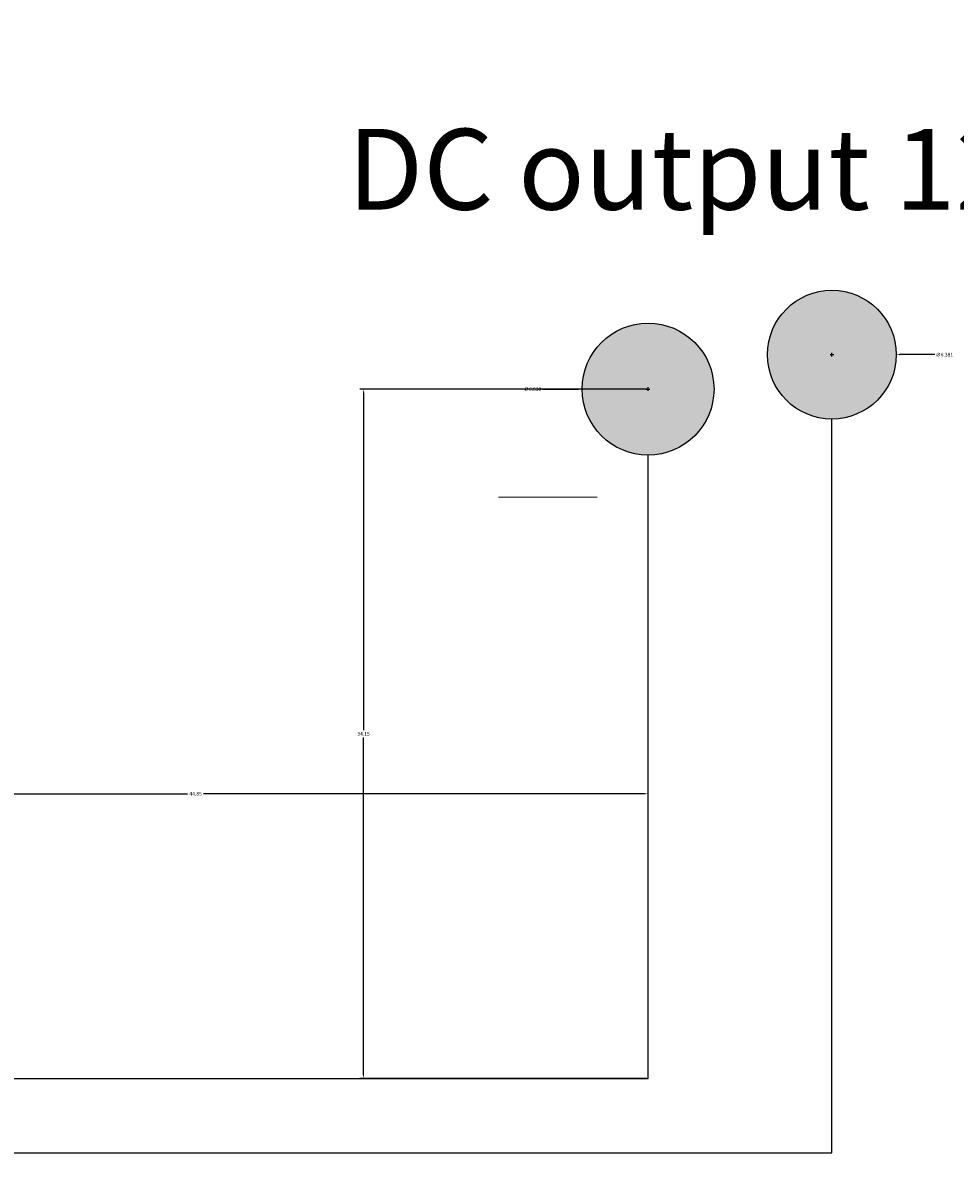
# Model space of a CAD drawing. Units: millimetres. Extents: x -8 to 285, y 5 to 221.
# Tile 9 of 30: x 84 to 130, y 56 to 113. Entities that reach past the tile are written whole.
import ezdxf

# ---------------------------------------------------------------- set-up
doc = ezdxf.new("R2010")
doc.units = ezdxf.units.MM
for name, color, linetype, lineweight in [('A-ANNO-DIMS', 2, 'Continuous', 18), ('E-ANNO-SYMB', 7, 'Continuous', 18), ('E-ANNO-TEXT', 7, 'Continuous', 18), ('E-EQPM-PATT', 252, 'Continuous', 13), ('E-POWR-DC-NEG', 3, 'Continuous', 25), ('E-POWR-LOAD', 7, 'Continuous', 25)]:
    doc.layers.add(name, color=color, linetype=linetype, lineweight=lineweight)
doc.layers.add('E-POWR-DC-POS', color=30, linetype='Continuous', lineweight=25, true_color=0xf26722)
doc.styles.get("Standard").update_dxf_attribs({"font": 'arial.ttf'})
doc.dimstyles.get("Standard").update_dxf_attribs({"dimtxt": 0.18, "dimasz": 0.18, "dimexe": 0.18, "dimexo": 0.0625, "dimgap": 0.09, "dimtad": 0, "dimtih": 1, "dimtoh": 1, "dimdec": 4, "dimzin": 0, "dimdsep": 46, "dimtxsty": 'Standard', "dimcen": 0.09, "dimadec": 0, "dimazin": 0, "dimtfac": 1, "dimtdec": 4, "dimtofl": 0, "dimtmove": 0, "dimatfit": 3, "dimfxl": 1, "dimtolj": 1, "dimtzin": 0, "dimarcsym": 0})

# ---------------------------------------------------------------- blocks, each defined once
blk = doc.blocks.new('*D10')
at = {"layer": 'A-ANNO-DIMS', "color": 0, "lineweight": -2, "transparency": 16777216}
for p, q in [((145.103, 206.457), (-7.608, 206.457)), ((-7.428, 206.277), (-7.428, 113.161)), ((-7.428, 19.682), (-7.428, 112.797)), ((30.453, 19.502), (-7.608, 19.502))]:
    blk.add_line(p, q, dxfattribs=at)
at = {"layer": 'A-ANNO-DIMS', "color": 0, "transparency": 16777216}
for points in [[(-7.458, 206.277), (-7.398, 206.277), (-7.428, 206.457)], [(-7.458, 19.682), (-7.398, 19.682), (-7.428, 19.502)]]:
    blk.add_solid(points, dxfattribs=at)
at = {"layer": 'Defpoints', "color": 0, "transparency": 16777216}
for p in [(-7.428, 206.457), (145.165, 206.457), (30.516, 19.502)]:
    blk.add_point(p, dxfattribs=at)
at = {"layer": 'A-ANNO-DIMS', "color": 0, "transparency": 16777216, "insert": (-7.428, 112.979), "char_height": 0.18, "attachment_point": 5}
blk.add_mtext('\\A1;186.95', dxfattribs=at)
blk = doc.blocks.new('*D25')
at = {"layer": 'A-ANNO-DIMS', "color": 0, "lineweight": -2, "transparency": 16777216}
for p, q in [((70.172, 60.759), (70.172, 74.977)), ((70.352, 74.797), (92.199, 74.797)), ((114.842, 74.797), (92.995, 74.797)), ((115.022, 60.759), (115.022, 74.977))]:
    blk.add_line(p, q, dxfattribs=at)
at = {"layer": 'A-ANNO-DIMS', "color": 0, "transparency": 16777216}
for points in [[(70.352, 74.827), (70.352, 74.767), (70.172, 74.797)], [(114.842, 74.827), (114.842, 74.767), (115.022, 74.797)]]:
    blk.add_solid(points, dxfattribs=at)
at = {"layer": 'Defpoints', "color": 0, "transparency": 16777216}
for p in [(115.022, 74.797), (70.172, 60.697), (115.022, 60.697)]:
    blk.add_point(p, dxfattribs=at)
at = {"layer": 'A-ANNO-DIMS', "color": 0, "transparency": 16777216, "insert": (92.597, 74.797), "char_height": 0.18, "attachment_point": 5}
blk.add_mtext('\\A1;44.85', dxfattribs=at)
blk = doc.blocks.new('*D26')
at = {"layer": 'A-ANNO-DIMS', "color": 0, "lineweight": -2, "transparency": 16777216}
for p, q in [((114.96, 94.844), (100.742, 94.844)), ((100.922, 94.664), (100.922, 77.953)), ((100.922, 60.877), (100.922, 77.589)), ((114.96, 60.697), (100.742, 60.697))]:
    blk.add_line(p, q, dxfattribs=at)
at = {"layer": 'A-ANNO-DIMS', "color": 0, "transparency": 16777216}
for points in [[(100.892, 94.664), (100.952, 94.664), (100.922, 94.844)], [(100.892, 60.877), (100.952, 60.877), (100.922, 60.697)]]:
    blk.add_solid(points, dxfattribs=at)
at = {"layer": 'Defpoints', "color": 0, "transparency": 16777216}
for p in [(100.922, 94.844), (115.022, 94.844), (115.022, 60.697)]:
    blk.add_point(p, dxfattribs=at)
at = {"layer": 'A-ANNO-DIMS', "color": 0, "transparency": 16777216, "insert": (100.922, 77.771), "char_height": 0.18, "attachment_point": 5}
blk.add_mtext('\\A1;34.15', dxfattribs=at)
blk = doc.blocks.new('*D35')
at = {"layer": 'A-ANNO-DIMS', "color": 0, "lineweight": -2, "transparency": 16777216}
for p, q in [((109.792, 94.844), (111.573, 94.844)), ((114.932, 94.844), (115.112, 94.844)), ((115.022, 94.754), (115.022, 94.934))]:
    blk.add_line(p, q, dxfattribs=at)
at = {"layer": 'A-ANNO-DIMS', "color": 0, "transparency": 16777216}
blk.add_solid([(111.573, 94.874), (111.573, 94.814), (111.753, 94.844)], dxfattribs=at)
at = {"layer": 'Defpoints', "color": 0, "transparency": 16777216}
for p in [(111.753, 94.844), (118.292, 94.845)]:
    blk.add_point(p, dxfattribs=at)
at = {"layer": 'A-ANNO-DIMS', "color": 0, "transparency": 16777216, "insert": (109.3, 94.844), "char_height": 0.18, "attachment_point": 5}
blk.add_mtext('\\A1;∅6.538', dxfattribs=at)
blk = doc.blocks.new('*D36')
at = {"layer": 'A-ANNO-DIMS', "color": 0, "lineweight": -2, "transparency": 16777216}
for p, q in [((124.044, 96.551), (124.224, 96.551)), ((124.134, 96.461), (124.134, 96.641)), ((129.239, 96.551), (127.504, 96.551))]:
    blk.add_line(p, q, dxfattribs=at)
at = {"layer": 'A-ANNO-DIMS', "color": 0, "transparency": 16777216}
blk.add_solid([(127.504, 96.581), (127.504, 96.521), (127.324, 96.551)], dxfattribs=at)
at = {"layer": 'Defpoints', "color": 0, "transparency": 16777216}
for p in [(120.944, 96.552), (127.324, 96.551)]:
    blk.add_point(p, dxfattribs=at)
at = {"layer": 'A-ANNO-DIMS', "color": 0, "transparency": 16777216, "insert": (129.713, 96.551), "char_height": 0.18, "attachment_point": 5}
blk.add_mtext('\\A1;∅6.381', dxfattribs=at)

msp = doc.modelspace()

# ---------------------------------------------------------------- hatches: boundary and pattern name
at = {"layer": 'E-EQPM-PATT'}
h = msp.add_hatch(color=256, dxfattribs=at)
h.set_gradient(color1=(248, 153, 30), color2=(248, 153, 30), tint=1)
h.paths.add_polyline_path([(111.7534, 94.8444, 1), (118.2915, 94.8444, 1)])
h.paths.add_polyline_path([(127.3244, 96.5513, 1), (120.9436, 96.5513, 1)])
h = msp.add_hatch(color=256, dxfattribs=at)
h.set_gradient(color1=(0, 255, 0), color2=(0, 255, 0), tint=1)
h.paths.add_polyline_path([(118.2915, 94.8444, 1), (111.7534, 94.8444, 1)])

# ---------------------------------------------------------------- linework, layer by layer
at = {"layer": 'E-ANNO-SYMB'}
msp.add_line((107.608, 89.4839), (112.5018, 89.4839), dxfattribs=at)
at = {"layer": 'E-POWR-DC-NEG'}
msp.add_lwpolyline([(70.1717, 67.9064), (70.1717, 60.6968), (115.0224, 60.6968), (115.0224, 91.5754)], dxfattribs=at)
at = {"layer": 'E-POWR-DC-POS'}
msp.add_lwpolyline([(64.1717, 67.9064), (64.1717, 57.0172), (124.134, 57.0172), (124.134, 93.361)], dxfattribs=at)
at = {"layer": 'E-POWR-LOAD'}
for centre, radius in [((124.134, 96.5513), 3.1904), ((115.0224, 94.8444), 3.2691)]:
    msp.add_circle(centre, radius, dxfattribs=at)

# ---------------------------------------------------------------- texts
at = {"layer": 'E-ANNO-TEXT', "insert": (100.1263, 107.7354), "char_height": 4, "attachment_point": 1}
msp.add_mtext_dynamic_manual_height_columns('DC output 12v DC load', width=65.111825, gutter_width=12.5, heights=[0], dxfattribs=at)

# ---------------------------------------------------------------- dimensions: what is measured, and where the dimension line sits
at = {"layer": 'A-ANNO-DIMS'}
for base, p1, p2, picture, middle in [((-7.4275, 206.4568), (30.516, 19.502), (145.1651, 206.4568), '*D10', (-7.4275, 112.9794)), ((100.9224, 94.8444), (115.0224, 60.6968), (115.0224, 94.8444), '*D26', (100.9224, 77.7706))]:
    dim = msp.add_linear_dim(base=base, p1=p1, p2=p2, angle=90, dimstyle='Standard', override={"dimdec": 2, "dimlfac": 1, "dimrnd": 0, "dimzin": 0, "dimdsep": 46, "dimlunit": 2}, dxfattribs=at)
    dim.commit()
    dim.dimension.update_dxf_attribs({"geometry": picture, "text_midpoint": middle})
for p1, p2, picture, middle in [((120.9436, 96.5517), (127.3244, 96.551), '*D36', (129.2386, 96.5508)), ((118.2915, 94.8449), (111.7534, 94.844), '*D35', (109.7919, 94.8437))]:
    dim = msp.add_diameter_dim_2p(p1=p1, p2=p2, dimstyle='Standard', override={"dimdec": 3, "dimlfac": 1, "dimrnd": 0, "dimzin": 0, "dimdsep": 46, "dimlunit": 2}, dxfattribs=at)
    dim.commit()
    dim.dimension.update_dxf_attribs({"geometry": picture, "text_midpoint": middle, "dimtype": 163})
dim = msp.add_linear_dim(base=(115.0224, 74.7968), p1=(70.1717, 60.6968), p2=(115.0224, 60.6968), dimstyle='Standard', override={"dimdec": 2, "dimlfac": 1, "dimrnd": 0, "dimzin": 0, "dimdsep": 46, "dimlunit": 2}, dxfattribs=at)
dim.commit()
dim.dimension.update_dxf_attribs({"geometry": '*D25', "text_midpoint": (92.597, 74.7968)})

doc.saveas('drawing.dxf')
